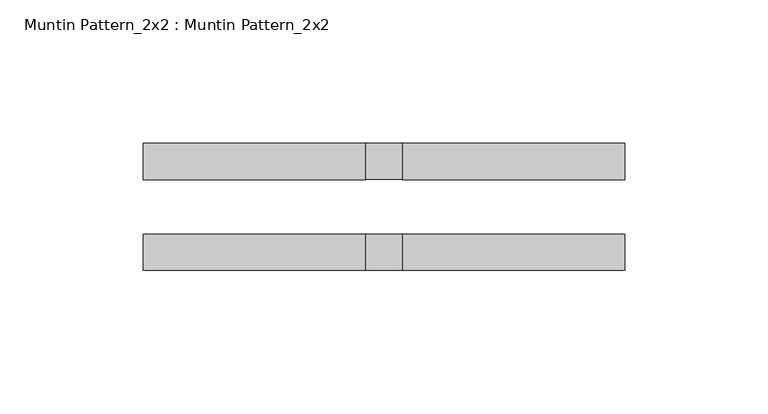
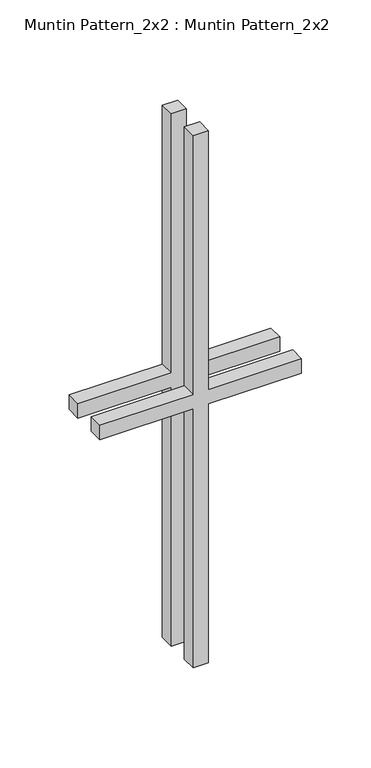
"""IFC4 building model written with IfcOpenShell, lengths in millimetres: proxy geometry, Muntin Pattern_2x2 : Muntin Pattern_2x2."""

from ifc_helpers import new_model, si_unit, frame, origin, place, context, project, spatial, polyline, outline, extrude, source, transform, mapped, element, save


def muntin_pattern_2x2_muntin_pattern_2x2_0961b91c(model_context):
    return source(origin(), model_context, "Body", "SweptSolid", [
        extrude(outline(polyline([(241.3, -6.35), (241.3, -84.1375), (228.6, -84.1375), (228.6, -6.35), (0.0, -6.35), (0.0, 6.35), (228.6, 6.35), (228.6, 84.1375), (241.3, 84.1375), (241.3, 6.35), (469.9, 6.35), (469.9, -6.35), (241.3, -6.35)])), frame((0.0, 9.525, 0.0), z_axis=(0.0, 1.0, 0.0), x_axis=(0.0, 0.0, 1.0)), (0.0, 0.0, 1.0), 12.7),
        extrude(outline(polyline([(241.3, -6.35), (241.3, -84.1375), (228.6, -84.1375), (228.6, -6.35), (0.0, -6.35), (0.0, 6.35), (228.6, 6.35), (228.6, 84.1375), (241.3, 84.1375), (241.3, 6.35), (469.9, 6.35), (469.9, -6.35), (241.3, -6.35)])), frame((0.0, -22.225, 0.0), z_axis=(0.0, 1.0, 0.0), x_axis=(0.0, 0.0, 1.0)), (0.0, 0.0, 1.0), 12.7),
    ])


if __name__ == "__main__":
    model = new_model("IFC4")
    model_context = context("Model", 3, world=origin())
    ifc_project = project(units=[si_unit("LENGTHUNIT", "METRE", prefix="MILLI")], contexts=[model_context])
    site = spatial("IfcSite", under=ifc_project)
    building = spatial("IfcBuilding", under=site)
    placement = place(None, origin())
    muntin_pattern_2x2_muntin_pattern_2x2_shape = muntin_pattern_2x2_muntin_pattern_2x2_0961b91c(model_context)
    element("IfcBuildingElementProxy", 1, Name="Muntin Pattern_2x2 : Muntin Pattern_2x2", ObjectType="Muntin Pattern_2x2 : Muntin Pattern_2x2", at=placement, inside=building, context=model_context, shape_type="MappedRepresentation", body=[
        mapped(muntin_pattern_2x2_muntin_pattern_2x2_shape, transform((0.0, 0.0, 0.0), x_axis=(1.0, 0.0, 0.0), y_axis=(0.0, 1.0, 0.0), z_axis=(0.0, 0.0, 1.0))),
    ])
    save(model, "model.ifc")

# Revit data of these elements
# Type "Muntin Pattern_2x2 : Muntin Pattern_2x2"
#   Width [instance default] = 4' - 0"
#   Thickness = 0' - 0 1/2"
#   Height [instance default] = 4' - 0"
#   Distance = 0' - 0 3/4"
#   Interior Material [instance default] = none
#   Exterior Material [instance default] = none
#   Default Elevation = 0
# Element 1 (IfcBuildingElementProxy, "Muntin Pattern_2x2 : Muntin Pattern_2x2")
#   Width = 0' - 6 5/8"
#   Height = 1' - 6 1/2"
#   Interior Material = Wood - Stained
#   Exterior Material = Clad - White
#   Materials on its faces: "Clad - White", "Wood - Stained"
# Materials
#   "Clad - White": class "Wood", colour RGB 242 242 238, transparency 0, Cost = 0
#   "Wood - Stained": class "Wood", colour RGB 224 178 126, transparency 0, Cost = 0
